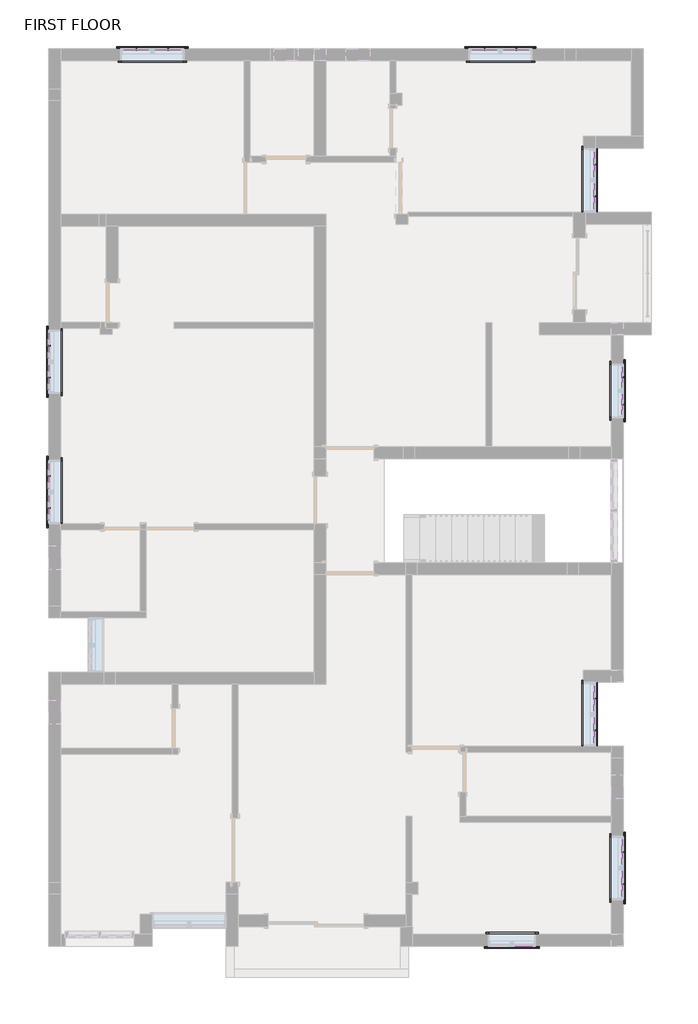
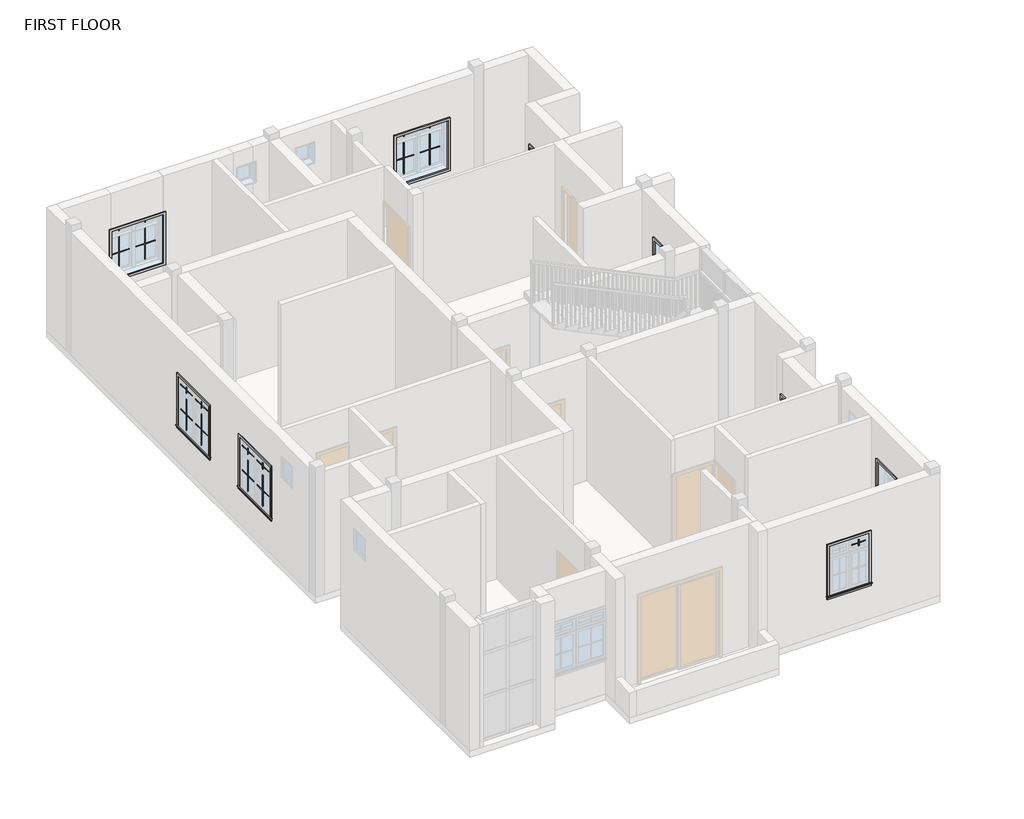
# One storey, part 6 of 6: 51 proxies.
"""IFC4 building model written with IfcOpenShell, lengths in millimetres."""

from ifc_helpers import new_model, si_unit, origin, place, context, project, spatial, transform, mapped, element, save
from components import muntin_pattern_2x2_muntin_pattern_2x2_2357e71d, muntin_pattern_2x2_muntin_pattern_2x2_302d8f29, muntin_pattern_2x2_muntin_pattern_2x2_3df65231, muntin_pattern_2x2_muntin_pattern_2x2_4af9dbf3, muntin_pattern_2x2_muntin_pattern_2x2_972acb6d, muntin_pattern_2x2_muntin_pattern_2x2_4879a4f3, muntin_pattern_2x2_muntin_pattern_2x2_604ffb00, trim_window_exterior_flat_with_sill_7cfdd449, trim_window_exterior_flat_with_sill_29d7a895, trim_window_exterior_flat_with_sill_e4b28ec3, trim_window_interior_flat_picture_frame_f1e0b15b, trim_window_interior_flat_picture_frame_56711e78, trim_window_interior_flat_picture_frame_39ff4276

model = new_model("IFC4")

# Units and contexts
model_context = context("Model", 3, world=origin())
ifc_project = project(units=[si_unit("LENGTHUNIT", "METRE", prefix="MILLI")], contexts=[model_context])

# Site, building, storey
site = spatial("IfcSite", under=ifc_project)
building = spatial("IfcBuilding", under=site)
storey = spatial("IfcBuildingStorey", under=building, Name="FIRST FLOOR", Elevation=3200.4)

# Proxies
placement = place(None, origin())
muntin_pattern_2x2_muntin_pattern_2x2_shape = muntin_pattern_2x2_muntin_pattern_2x2_2357e71d(model_context)
element("IfcBuildingElementProxy", 1, Name="Muntin Pattern_2x2 : Muntin Pattern_2x2", ObjectType="Muntin Pattern_2x2 : Muntin Pattern_2x2", at=placement, inside=storey, context=model_context, shape_type="MappedRepresentation", body=[
    mapped(muntin_pattern_2x2_muntin_pattern_2x2_shape, transform((-5090.4990981, 9290.6537587, 4184.65), x_axis=(1.0, 0.0, 0.0), y_axis=(0.0, 1.0, 0.0), z_axis=(0.0, 0.0, 1.0))),
])
element("IfcBuildingElementProxy", 2, Name="Muntin Pattern_2x2 : Muntin Pattern_2x2", ObjectType="Muntin Pattern_2x2 : Muntin Pattern_2x2", at=placement, inside=storey, context=model_context, shape_type="MappedRepresentation", body=[
    mapped(muntin_pattern_2x2_muntin_pattern_2x2_shape, transform((3661.3884019, 7088.7912587, 4184.65), x_axis=(0.0, -1.0, 0.0), y_axis=(1.0, 0.0, 0.0), z_axis=(0.0, 0.0, 1.0))),
])
element("IfcBuildingElementProxy", 3, Name="Muntin Pattern_2x2 : Muntin Pattern_2x2", ObjectType="Muntin Pattern_2x2 : Muntin Pattern_2x2", at=placement, inside=storey, context=model_context, shape_type="MappedRepresentation", body=[
    mapped(muntin_pattern_2x2_muntin_pattern_2x2_shape, transform((3661.3884019, -3096.6087413, 4184.65), x_axis=(0.0, -1.0, 0.0), y_axis=(1.0, 0.0, 0.0), z_axis=(0.0, 0.0, 1.0))),
])
element("IfcBuildingElementProxy", 4, Name="Muntin Pattern_2x2 : Muntin Pattern_2x2", ObjectType="Muntin Pattern_2x2 : Muntin Pattern_2x2", at=placement, inside=storey, context=model_context, shape_type="MappedRepresentation", body=[
    mapped(muntin_pattern_2x2_muntin_pattern_2x2_shape, transform((4194.7884019, -6025.7255734, 4184.65), x_axis=(0.0, -1.0, 0.0), y_axis=(1.0, 0.0, 0.0), z_axis=(0.0, 0.0, 1.0))),
])
element("IfcBuildingElementProxy", 5, Name="Muntin Pattern_2x2 : Muntin Pattern_2x2", ObjectType="Muntin Pattern_2x2 : Muntin Pattern_2x2", at=placement, inside=storey, context=model_context, shape_type="MappedRepresentation", body=[
    mapped(muntin_pattern_2x2_muntin_pattern_2x2_shape, transform((-6758.9615981, 538.7662587, 4184.65), x_axis=(0.0, 1.0, 0.0), y_axis=(-1.0, 0.0, 0.0), z_axis=(0.0, 0.0, 1.0))),
])
element("IfcBuildingElementProxy", 6, Name="Muntin Pattern_2x2 : Muntin Pattern_2x2", ObjectType="Muntin Pattern_2x2 : Muntin Pattern_2x2", at=placement, inside=storey, context=model_context, shape_type="MappedRepresentation", body=[
    mapped(muntin_pattern_2x2_muntin_pattern_2x2_shape, transform((-6758.9615981, 3024.5447861, 4184.65), x_axis=(0.0, 1.0, 0.0), y_axis=(-1.0, 0.0, 0.0), z_axis=(0.0, 0.0, 1.0))),
])
element("IfcBuildingElementProxy", 7, Name="Muntin Pattern_2x2 : Muntin Pattern_2x2", ObjectType="Muntin Pattern_2x2 : Muntin Pattern_2x2", at=placement, inside=storey, context=model_context, shape_type="MappedRepresentation", body=[
    mapped(muntin_pattern_2x2_muntin_pattern_2x2_shape, transform((1554.8452655, 9290.6537587, 4184.65), x_axis=(1.0, 0.0, 0.0), y_axis=(0.0, 1.0, 0.0), z_axis=(0.0, 0.0, 1.0))),
])
muntin_pattern_2x2_muntin_pattern_2x2_2_shape = muntin_pattern_2x2_muntin_pattern_2x2_302d8f29(model_context)
element("IfcBuildingElementProxy", 8, Name="Muntin Pattern_2x2 : Muntin Pattern_2x2", ObjectType="Muntin Pattern_2x2 : Muntin Pattern_2x2", at=placement, inside=storey, context=model_context, shape_type="MappedRepresentation", body=[
    mapped(muntin_pattern_2x2_muntin_pattern_2x2_2_shape, transform((-4484.0740981, 9290.6537587, 4184.65), x_axis=(-1.0, 0.0, 0.0), y_axis=(0.0, -1.0, 0.0), z_axis=(0.0, 0.0, 1.0))),
])
element("IfcBuildingElementProxy", 9, Name="Muntin Pattern_2x2 : Muntin Pattern_2x2", ObjectType="Muntin Pattern_2x2 : Muntin Pattern_2x2", at=placement, inside=storey, context=model_context, shape_type="MappedRepresentation", body=[
    mapped(muntin_pattern_2x2_muntin_pattern_2x2_2_shape, transform((3661.3884019, 6482.3662587, 4184.65), x_axis=(0.0, 1.0, 0.0), y_axis=(-1.0, 0.0, 0.0), z_axis=(0.0, 0.0, 1.0))),
])
element("IfcBuildingElementProxy", 10, Name="Muntin Pattern_2x2 : Muntin Pattern_2x2", ObjectType="Muntin Pattern_2x2 : Muntin Pattern_2x2", at=placement, inside=storey, context=model_context, shape_type="MappedRepresentation", body=[
    mapped(muntin_pattern_2x2_muntin_pattern_2x2_2_shape, transform((3661.3884019, -3703.0337413, 4184.65), x_axis=(0.0, 1.0, 0.0), y_axis=(-1.0, 0.0, 0.0), z_axis=(0.0, 0.0, 1.0))),
])
element("IfcBuildingElementProxy", 11, Name="Muntin Pattern_2x2 : Muntin Pattern_2x2", ObjectType="Muntin Pattern_2x2 : Muntin Pattern_2x2", at=placement, inside=storey, context=model_context, shape_type="MappedRepresentation", body=[
    mapped(muntin_pattern_2x2_muntin_pattern_2x2_2_shape, transform((4194.7884019, -6632.1505734, 4184.65), x_axis=(0.0, 1.0, 0.0), y_axis=(-1.0, 0.0, 0.0), z_axis=(0.0, 0.0, 1.0))),
])
element("IfcBuildingElementProxy", 12, Name="Muntin Pattern_2x2 : Muntin Pattern_2x2", ObjectType="Muntin Pattern_2x2 : Muntin Pattern_2x2", at=placement, inside=storey, context=model_context, shape_type="MappedRepresentation", body=[
    mapped(muntin_pattern_2x2_muntin_pattern_2x2_2_shape, transform((-6758.9615981, 1145.1912587, 4184.65), x_axis=(0.0, -1.0, 0.0), y_axis=(1.0, 0.0, 0.0), z_axis=(0.0, 0.0, 1.0))),
])
element("IfcBuildingElementProxy", 13, Name="Muntin Pattern_2x2 : Muntin Pattern_2x2", ObjectType="Muntin Pattern_2x2 : Muntin Pattern_2x2", at=placement, inside=storey, context=model_context, shape_type="MappedRepresentation", body=[
    mapped(muntin_pattern_2x2_muntin_pattern_2x2_2_shape, transform((-6758.9615981, 3630.9697861, 4184.65), x_axis=(0.0, -1.0, 0.0), y_axis=(1.0, 0.0, 0.0), z_axis=(0.0, 0.0, 1.0))),
])
element("IfcBuildingElementProxy", 14, Name="Muntin Pattern_2x2 : Muntin Pattern_2x2", ObjectType="Muntin Pattern_2x2 : Muntin Pattern_2x2", at=placement, inside=storey, context=model_context, shape_type="MappedRepresentation", body=[
    mapped(muntin_pattern_2x2_muntin_pattern_2x2_2_shape, transform((2161.2702655, 9290.6537587, 4184.65), x_axis=(-1.0, 0.0, 0.0), y_axis=(0.0, -1.0, 0.0), z_axis=(0.0, 0.0, 1.0))),
])
muntin_pattern_2x2_muntin_pattern_2x2_3_shape = muntin_pattern_2x2_muntin_pattern_2x2_3df65231(model_context)
element("IfcBuildingElementProxy", 15, Name="Muntin Pattern_2x2 : Muntin Pattern_2x2", ObjectType="Muntin Pattern_2x2 : Muntin Pattern_2x2", at=placement, inside=storey, context=model_context, shape_type="MappedRepresentation", body=[
    mapped(muntin_pattern_2x2_muntin_pattern_2x2_3_shape, transform((-4484.0740981, 9290.6537587, 5099.05), x_axis=(-1.0, 0.0, 0.0), y_axis=(0.0, -1.0, 0.0), z_axis=(0.0, 0.0, 1.0))),
])
element("IfcBuildingElementProxy", 16, Name="Muntin Pattern_2x2 : Muntin Pattern_2x2", ObjectType="Muntin Pattern_2x2 : Muntin Pattern_2x2", at=placement, inside=storey, context=model_context, shape_type="MappedRepresentation", body=[
    mapped(muntin_pattern_2x2_muntin_pattern_2x2_3_shape, transform((-5090.4990981, 9290.6537587, 5099.05), x_axis=(-1.0, 0.0, 0.0), y_axis=(0.0, -1.0, 0.0), z_axis=(0.0, 0.0, 1.0))),
])
element("IfcBuildingElementProxy", 17, Name="Muntin Pattern_2x2 : Muntin Pattern_2x2", ObjectType="Muntin Pattern_2x2 : Muntin Pattern_2x2", at=placement, inside=storey, context=model_context, shape_type="MappedRepresentation", body=[
    mapped(muntin_pattern_2x2_muntin_pattern_2x2_3_shape, transform((3661.3884019, 6482.3662587, 5099.05), x_axis=(0.0, 1.0, 0.0), y_axis=(-1.0, 0.0, 0.0), z_axis=(0.0, 0.0, 1.0))),
])
element("IfcBuildingElementProxy", 18, Name="Muntin Pattern_2x2 : Muntin Pattern_2x2", ObjectType="Muntin Pattern_2x2 : Muntin Pattern_2x2", at=placement, inside=storey, context=model_context, shape_type="MappedRepresentation", body=[
    mapped(muntin_pattern_2x2_muntin_pattern_2x2_3_shape, transform((3661.3884019, 7088.7912587, 5099.05), x_axis=(0.0, 1.0, 0.0), y_axis=(-1.0, 0.0, 0.0), z_axis=(0.0, 0.0, 1.0))),
])
element("IfcBuildingElementProxy", 19, Name="Muntin Pattern_2x2 : Muntin Pattern_2x2", ObjectType="Muntin Pattern_2x2 : Muntin Pattern_2x2", at=placement, inside=storey, context=model_context, shape_type="MappedRepresentation", body=[
    mapped(muntin_pattern_2x2_muntin_pattern_2x2_3_shape, transform((3661.3884019, -3703.0337413, 5099.05), x_axis=(0.0, 1.0, 0.0), y_axis=(-1.0, 0.0, 0.0), z_axis=(0.0, 0.0, 1.0))),
])
element("IfcBuildingElementProxy", 20, Name="Muntin Pattern_2x2 : Muntin Pattern_2x2", ObjectType="Muntin Pattern_2x2 : Muntin Pattern_2x2", at=placement, inside=storey, context=model_context, shape_type="MappedRepresentation", body=[
    mapped(muntin_pattern_2x2_muntin_pattern_2x2_3_shape, transform((3661.3884019, -3096.6087413, 5099.05), x_axis=(0.0, 1.0, 0.0), y_axis=(-1.0, 0.0, 0.0), z_axis=(0.0, 0.0, 1.0))),
])
element("IfcBuildingElementProxy", 21, Name="Muntin Pattern_2x2 : Muntin Pattern_2x2", ObjectType="Muntin Pattern_2x2 : Muntin Pattern_2x2", at=placement, inside=storey, context=model_context, shape_type="MappedRepresentation", body=[
    mapped(muntin_pattern_2x2_muntin_pattern_2x2_3_shape, transform((4194.7884019, -6632.1505734, 5099.05), x_axis=(0.0, 1.0, 0.0), y_axis=(-1.0, 0.0, 0.0), z_axis=(0.0, 0.0, 1.0))),
])
element("IfcBuildingElementProxy", 22, Name="Muntin Pattern_2x2 : Muntin Pattern_2x2", ObjectType="Muntin Pattern_2x2 : Muntin Pattern_2x2", at=placement, inside=storey, context=model_context, shape_type="MappedRepresentation", body=[
    mapped(muntin_pattern_2x2_muntin_pattern_2x2_3_shape, transform((4194.7884019, -6025.7255734, 5099.05), x_axis=(0.0, 1.0, 0.0), y_axis=(-1.0, 0.0, 0.0), z_axis=(0.0, 0.0, 1.0))),
])
element("IfcBuildingElementProxy", 23, Name="Muntin Pattern_2x2 : Muntin Pattern_2x2", ObjectType="Muntin Pattern_2x2 : Muntin Pattern_2x2", at=placement, inside=storey, context=model_context, shape_type="MappedRepresentation", body=[
    mapped(muntin_pattern_2x2_muntin_pattern_2x2_3_shape, transform((-6758.9615981, 1145.1912587, 5099.05), x_axis=(0.0, -1.0, 0.0), y_axis=(1.0, 0.0, 0.0), z_axis=(0.0, 0.0, 1.0))),
])
element("IfcBuildingElementProxy", 24, Name="Muntin Pattern_2x2 : Muntin Pattern_2x2", ObjectType="Muntin Pattern_2x2 : Muntin Pattern_2x2", at=placement, inside=storey, context=model_context, shape_type="MappedRepresentation", body=[
    mapped(muntin_pattern_2x2_muntin_pattern_2x2_3_shape, transform((-6758.9615981, 538.7662587, 5099.05), x_axis=(0.0, -1.0, 0.0), y_axis=(1.0, 0.0, 0.0), z_axis=(0.0, 0.0, 1.0))),
])
element("IfcBuildingElementProxy", 25, Name="Muntin Pattern_2x2 : Muntin Pattern_2x2", ObjectType="Muntin Pattern_2x2 : Muntin Pattern_2x2", at=placement, inside=storey, context=model_context, shape_type="MappedRepresentation", body=[
    mapped(muntin_pattern_2x2_muntin_pattern_2x2_3_shape, transform((-6758.9615981, 3630.9697861, 5099.05), x_axis=(0.0, -1.0, 0.0), y_axis=(1.0, 0.0, 0.0), z_axis=(0.0, 0.0, 1.0))),
])
element("IfcBuildingElementProxy", 26, Name="Muntin Pattern_2x2 : Muntin Pattern_2x2", ObjectType="Muntin Pattern_2x2 : Muntin Pattern_2x2", at=placement, inside=storey, context=model_context, shape_type="MappedRepresentation", body=[
    mapped(muntin_pattern_2x2_muntin_pattern_2x2_3_shape, transform((-6758.9615981, 3024.5447861, 5099.05), x_axis=(0.0, -1.0, 0.0), y_axis=(1.0, 0.0, 0.0), z_axis=(0.0, 0.0, 1.0))),
])
element("IfcBuildingElementProxy", 27, Name="Muntin Pattern_2x2 : Muntin Pattern_2x2", ObjectType="Muntin Pattern_2x2 : Muntin Pattern_2x2", at=placement, inside=storey, context=model_context, shape_type="MappedRepresentation", body=[
    mapped(muntin_pattern_2x2_muntin_pattern_2x2_3_shape, transform((2161.2702655, 9290.6537587, 5099.05), x_axis=(-1.0, 0.0, 0.0), y_axis=(0.0, -1.0, 0.0), z_axis=(0.0, 0.0, 1.0))),
])
element("IfcBuildingElementProxy", 28, Name="Muntin Pattern_2x2 : Muntin Pattern_2x2", ObjectType="Muntin Pattern_2x2 : Muntin Pattern_2x2", at=placement, inside=storey, context=model_context, shape_type="MappedRepresentation", body=[
    mapped(muntin_pattern_2x2_muntin_pattern_2x2_3_shape, transform((1554.8452655, 9290.6537587, 5099.05), x_axis=(-1.0, 0.0, 0.0), y_axis=(0.0, -1.0, 0.0), z_axis=(0.0, 0.0, 1.0))),
])
muntin_pattern_2x2_muntin_pattern_2x2_4_shape = muntin_pattern_2x2_muntin_pattern_2x2_4af9dbf3(model_context)
element("IfcBuildingElementProxy", 29, Name="Muntin Pattern_2x2 : Muntin Pattern_2x2", ObjectType="Muntin Pattern_2x2 : Muntin Pattern_2x2", at=placement, inside=storey, context=model_context, shape_type="MappedRepresentation", body=[
    mapped(muntin_pattern_2x2_muntin_pattern_2x2_4_shape, transform((4194.7884019, 3031.1412587, 4184.65), x_axis=(0.0, -1.0, 0.0), y_axis=(1.0, 0.0, 0.0), z_axis=(0.0, 0.0, 1.0))),
])
muntin_pattern_2x2_muntin_pattern_2x2_5_shape = muntin_pattern_2x2_muntin_pattern_2x2_972acb6d(model_context)
element("IfcBuildingElementProxy", 30, Name="Muntin Pattern_2x2 : Muntin Pattern_2x2", ObjectType="Muntin Pattern_2x2 : Muntin Pattern_2x2", at=placement, inside=storey, context=model_context, shape_type="MappedRepresentation", body=[
    mapped(muntin_pattern_2x2_muntin_pattern_2x2_5_shape, transform((4194.7884019, 2513.6162587, 4184.65), x_axis=(0.0, 1.0, 0.0), y_axis=(-1.0, 0.0, 0.0), z_axis=(0.0, 0.0, 1.0))),
])
muntin_pattern_2x2_muntin_pattern_2x2_6_shape = muntin_pattern_2x2_muntin_pattern_2x2_4879a4f3(model_context)
element("IfcBuildingElementProxy", 31, Name="Muntin Pattern_2x2 : Muntin Pattern_2x2", ObjectType="Muntin Pattern_2x2 : Muntin Pattern_2x2", at=placement, inside=storey, context=model_context, shape_type="MappedRepresentation", body=[
    mapped(muntin_pattern_2x2_muntin_pattern_2x2_6_shape, transform((4194.7884019, 2513.6162587, 5099.05), x_axis=(0.0, 1.0, 0.0), y_axis=(-1.0, 0.0, 0.0), z_axis=(0.0, 0.0, 1.0))),
])
element("IfcBuildingElementProxy", 32, Name="Muntin Pattern_2x2 : Muntin Pattern_2x2", ObjectType="Muntin Pattern_2x2 : Muntin Pattern_2x2", at=placement, inside=storey, context=model_context, shape_type="MappedRepresentation", body=[
    mapped(muntin_pattern_2x2_muntin_pattern_2x2_6_shape, transform((4194.7884019, 3031.1412587, 5099.05), x_axis=(0.0, 1.0, 0.0), y_axis=(-1.0, 0.0, 0.0), z_axis=(0.0, 0.0, 1.0))),
])
muntin_pattern_2x2_muntin_pattern_2x2_7_shape = muntin_pattern_2x2_muntin_pattern_2x2_604ffb00(model_context)
element("IfcBuildingElementProxy", 33, Name="Muntin Pattern_2x2 : Muntin Pattern_2x2", ObjectType="Muntin Pattern_2x2 : Muntin Pattern_2x2", at=placement, inside=storey, context=model_context, shape_type="MappedRepresentation", body=[
    mapped(muntin_pattern_2x2_muntin_pattern_2x2_7_shape, transform((2304.0759019, -7809.8962413, 5099.05), x_axis=(1.0, 0.0, 0.0), y_axis=(0.0, 1.0, 0.0), z_axis=(0.0, 0.0, 1.0))),
])
trim_window_exterior_flat_with_sill_shape = trim_window_exterior_flat_with_sill_7cfdd449(model_context)
element("IfcBuildingElementProxy", 34, Name="Trim-Window-Exterior-Flat : with Sill", ObjectType="Trim-Window-Exterior-Flat : with Sill", at=placement, inside=storey, context=model_context, shape_type="MappedRepresentation", body=[
    mapped(trim_window_exterior_flat_with_sill_shape, transform((-4787.2865981, 9300.1787587, 5334.0), x_axis=(-1.0, 0.0, 0.0), y_axis=(0.0, 0.0, 1.0), z_axis=(0.0, 1.0, 0.0))),
])
element("IfcBuildingElementProxy", 35, Name="Trim-Window-Exterior-Flat : with Sill", ObjectType="Trim-Window-Exterior-Flat : with Sill", at=placement, inside=storey, context=model_context, shape_type="MappedRepresentation", body=[
    mapped(trim_window_exterior_flat_with_sill_shape, transform((3670.9134019, 6785.5787587, 5334.0), x_axis=(0.0, 1.0, 0.0), y_axis=(0.0, 0.0, 1.0), z_axis=(1.0, 0.0, 0.0))),
])
element("IfcBuildingElementProxy", 36, Name="Trim-Window-Exterior-Flat : with Sill", ObjectType="Trim-Window-Exterior-Flat : with Sill", at=placement, inside=storey, context=model_context, shape_type="MappedRepresentation", body=[
    mapped(trim_window_exterior_flat_with_sill_shape, transform((3670.9134019, -3399.8212413, 5334.0), x_axis=(0.0, 1.0, 0.0), y_axis=(0.0, 0.0, 1.0), z_axis=(1.0, 0.0, 0.0))),
])
element("IfcBuildingElementProxy", 37, Name="Trim-Window-Exterior-Flat : with Sill", ObjectType="Trim-Window-Exterior-Flat : with Sill", at=placement, inside=storey, context=model_context, shape_type="MappedRepresentation", body=[
    mapped(trim_window_exterior_flat_with_sill_shape, transform((4204.3134019, -6328.9380734, 5334.0), x_axis=(0.0, 1.0, 0.0), y_axis=(0.0, 0.0, 1.0), z_axis=(1.0, 0.0, 0.0))),
])
element("IfcBuildingElementProxy", 38, Name="Trim-Window-Exterior-Flat : with Sill", ObjectType="Trim-Window-Exterior-Flat : with Sill", at=placement, inside=storey, context=model_context, shape_type="MappedRepresentation", body=[
    mapped(trim_window_exterior_flat_with_sill_shape, transform((-6768.4865981, 841.9787587, 5334.0), x_axis=(0.0, -1.0, 0.0), y_axis=(0.0, 0.0, 1.0), z_axis=(-1.0, 0.0, 0.0))),
])
element("IfcBuildingElementProxy", 39, Name="Trim-Window-Exterior-Flat : with Sill", ObjectType="Trim-Window-Exterior-Flat : with Sill", at=placement, inside=storey, context=model_context, shape_type="MappedRepresentation", body=[
    mapped(trim_window_exterior_flat_with_sill_shape, transform((-6768.4865981, 3327.7572861, 5334.0), x_axis=(0.0, -1.0, 0.0), y_axis=(0.0, 0.0, 1.0), z_axis=(-1.0, 0.0, 0.0))),
])
element("IfcBuildingElementProxy", 40, Name="Trim-Window-Exterior-Flat : with Sill", ObjectType="Trim-Window-Exterior-Flat : with Sill", at=placement, inside=storey, context=model_context, shape_type="MappedRepresentation", body=[
    mapped(trim_window_exterior_flat_with_sill_shape, transform((1858.0577655, 9300.1787587, 5334.0), x_axis=(-1.0, 0.0, 0.0), y_axis=(0.0, 0.0, 1.0), z_axis=(0.0, 1.0, 0.0))),
])
trim_window_exterior_flat_with_sill_2_shape = trim_window_exterior_flat_with_sill_29d7a895(model_context)
element("IfcBuildingElementProxy", 41, Name="Trim-Window-Exterior-Flat : with Sill", ObjectType="Trim-Window-Exterior-Flat : with Sill", at=placement, inside=storey, context=model_context, shape_type="MappedRepresentation", body=[
    mapped(trim_window_exterior_flat_with_sill_2_shape, transform((4204.3134019, 2772.3787587, 5334.0), x_axis=(0.0, 1.0, 0.0), y_axis=(0.0, 0.0, 1.0), z_axis=(1.0, 0.0, 0.0))),
])
trim_window_exterior_flat_with_sill_3_shape = trim_window_exterior_flat_with_sill_e4b28ec3(model_context)
element("IfcBuildingElementProxy", 42, Name="Trim-Window-Exterior-Flat : with Sill", ObjectType="Trim-Window-Exterior-Flat : with Sill", at=placement, inside=storey, context=model_context, shape_type="MappedRepresentation", body=[
    mapped(trim_window_exterior_flat_with_sill_3_shape, transform((2077.0634019, -7819.4212413, 5334.0), x_axis=(1.0, 0.0, 0.0), y_axis=(0.0, 0.0, 1.0), z_axis=(0.0, -1.0, 0.0))),
])
trim_window_interior_flat_picture_frame_shape = trim_window_interior_flat_picture_frame_f1e0b15b(model_context)
element("IfcBuildingElementProxy", 43, Name="Trim-Window-Interior-Flat : Picture Frame", ObjectType="Trim-Window-Interior-Flat : Picture Frame", at=placement, inside=storey, context=model_context, shape_type="MappedRepresentation", body=[
    mapped(trim_window_interior_flat_picture_frame_shape, transform((-4787.2865981, 9071.5787587, 5334.0), x_axis=(1.0, 0.0, 0.0), y_axis=(0.0, 0.0, 1.0), z_axis=(0.0, -1.0, 0.0))),
])
element("IfcBuildingElementProxy", 44, Name="Trim-Window-Interior-Flat : Picture Frame", ObjectType="Trim-Window-Interior-Flat : Picture Frame", at=placement, inside=storey, context=model_context, shape_type="MappedRepresentation", body=[
    mapped(trim_window_interior_flat_picture_frame_shape, transform((3442.3134019, 6785.5787587, 5334.0), x_axis=(0.0, -1.0, 0.0), y_axis=(0.0, 0.0, 1.0), z_axis=(-1.0, 0.0, 0.0))),
])
element("IfcBuildingElementProxy", 45, Name="Trim-Window-Interior-Flat : Picture Frame", ObjectType="Trim-Window-Interior-Flat : Picture Frame", at=placement, inside=storey, context=model_context, shape_type="MappedRepresentation", body=[
    mapped(trim_window_interior_flat_picture_frame_shape, transform((3442.3134019, -3399.8212413, 5334.0), x_axis=(0.0, -1.0, 0.0), y_axis=(0.0, 0.0, 1.0), z_axis=(-1.0, 0.0, 0.0))),
])
element("IfcBuildingElementProxy", 46, Name="Trim-Window-Interior-Flat : Picture Frame", ObjectType="Trim-Window-Interior-Flat : Picture Frame", at=placement, inside=storey, context=model_context, shape_type="MappedRepresentation", body=[
    mapped(trim_window_interior_flat_picture_frame_shape, transform((3975.7134019, -6328.9380734, 5334.0), x_axis=(0.0, -1.0, 0.0), y_axis=(0.0, 0.0, 1.0), z_axis=(-1.0, 0.0, 0.0))),
])
element("IfcBuildingElementProxy", 47, Name="Trim-Window-Interior-Flat : Picture Frame", ObjectType="Trim-Window-Interior-Flat : Picture Frame", at=placement, inside=storey, context=model_context, shape_type="MappedRepresentation", body=[
    mapped(trim_window_interior_flat_picture_frame_shape, transform((-6539.8865981, 841.9787587, 5334.0), x_axis=(0.0, 1.0, 0.0), y_axis=(0.0, 0.0, 1.0), z_axis=(1.0, 0.0, 0.0))),
])
element("IfcBuildingElementProxy", 48, Name="Trim-Window-Interior-Flat : Picture Frame", ObjectType="Trim-Window-Interior-Flat : Picture Frame", at=placement, inside=storey, context=model_context, shape_type="MappedRepresentation", body=[
    mapped(trim_window_interior_flat_picture_frame_shape, transform((-6539.8865981, 3327.7572861, 5334.0), x_axis=(0.0, 1.0, 0.0), y_axis=(0.0, 0.0, 1.0), z_axis=(1.0, 0.0, 0.0))),
])
element("IfcBuildingElementProxy", 49, Name="Trim-Window-Interior-Flat : Picture Frame", ObjectType="Trim-Window-Interior-Flat : Picture Frame", at=placement, inside=storey, context=model_context, shape_type="MappedRepresentation", body=[
    mapped(trim_window_interior_flat_picture_frame_shape, transform((1858.0577655, 9071.5787587, 5334.0), x_axis=(1.0, 0.0, 0.0), y_axis=(0.0, 0.0, 1.0), z_axis=(0.0, -1.0, 0.0))),
])
trim_window_interior_flat_picture_frame_2_shape = trim_window_interior_flat_picture_frame_56711e78(model_context)
element("IfcBuildingElementProxy", 50, Name="Trim-Window-Interior-Flat : Picture Frame", ObjectType="Trim-Window-Interior-Flat : Picture Frame", at=placement, inside=storey, context=model_context, shape_type="MappedRepresentation", body=[
    mapped(trim_window_interior_flat_picture_frame_2_shape, transform((3975.7134019, 2772.3787587, 5334.0), x_axis=(0.0, -1.0, 0.0), y_axis=(0.0, 0.0, 1.0), z_axis=(-1.0, 0.0, 0.0))),
])
trim_window_interior_flat_picture_frame_3_shape = trim_window_interior_flat_picture_frame_39ff4276(model_context)
element("IfcBuildingElementProxy", 51, Name="Trim-Window-Interior-Flat : Picture Frame", ObjectType="Trim-Window-Interior-Flat : Picture Frame", at=placement, inside=storey, context=model_context, shape_type="MappedRepresentation", body=[
    mapped(trim_window_interior_flat_picture_frame_3_shape, transform((2077.0634019, -7590.8212413, 5334.0), x_axis=(-1.0, 0.0, 0.0), y_axis=(0.0, 0.0, 1.0), z_axis=(0.0, 1.0, 0.0))),
])

save(model, "model.ifc")

# Revit data of these elements
# Type "Muntin Pattern_2x2 : Muntin Pattern_2x2"
#   Width [instance default] = 4' - 0"
#   Thickness = 0' - 0 1/2"
#   Height [instance default] = 4' - 0"
#   Distance = 0' - 0 3/4"
#   Interior Material [instance default] = none
#   Exterior Material [instance default] = none
#   Default Elevation = 0
# Type "Trim-Window-Exterior-Flat : with Sill"
#   Trim Width = 0' - 2 1/4"
#   Trim Thickness_Picture Frame = 0' - 1 1/4"
#   Trim Thickness_with Sill = 0' - 0 3/4"
#   Sill Thickness = 0' - 1 1/4"
#   Opening Width [instance default] = 2' - 0"
#   Opening Height [instance default] = 3' - 0"
#   Default Elevation = 4' - 0"
#   Sill = yes
#   Picture Frame = no
#   Trim Material [instance default] = none
# Type "Trim-Window-Interior-Flat : Picture Frame"
#   Trim Thickness_Picture Frame = 0' - 1 1/4"
#   Trim Width = 0' - 2 1/4"
#   Trim Thickness_with Sill = 0' - 0 3/4"
#   Sill Thickness = 0' - 1 1/4"
#   Opening Width [instance default] = 2' - 0"
#   Opening Height [instance default] = 3' - 0"
#   Default Elevation = 4' - 0"
#   Sill = no
#   Picture Frame = yes
#   Trim Material [instance default] = none
# Elements 1, 2, 3, 4, 5, 6, 7, 8, 9, 10, 11, 12, 13, 14 (IfcBuildingElementProxy, "Muntin Pattern_2x2 : Muntin Pattern_2x2")
#   Width = 1' - 6 5/8"
#   Height = 2' - 6 1/2"
#   Interior Material = Wood - Stained
#   Exterior Material = Clad - White
#   Phase Created = New Construction
#   Materials on its faces: "Clad - White", "Wood - Stained"
# Elements 15, 16, 17, 18, 19, 20, 21, 22, 23, 24, 25, 26, 27, 28 (IfcBuildingElementProxy, "Muntin Pattern_2x2 : Muntin Pattern_2x2")
#   Width = 1' - 6 5/8"
#   Height = 0' - 6 1/2"
#   Interior Material = Wood - Stained
#   Exterior Material = Clad - White
#   Phase Created = New Construction
#   Materials on its faces: "Clad - White", "Wood - Stained"
# Elements 29, 30 (IfcBuildingElementProxy, "Muntin Pattern_2x2 : Muntin Pattern_2x2")
#   Width = 1' - 3 1/8"
#   Height = 2' - 6 1/2"
#   Interior Material = Wood - Stained
#   Exterior Material = Clad - White
#   Phase Created = New Construction
#   Materials on its faces: "Clad - White", "Wood - Stained"
# Elements 31, 32 (IfcBuildingElementProxy, "Muntin Pattern_2x2 : Muntin Pattern_2x2")
#   Width = 1' - 3 1/8"
#   Height = 0' - 6 1/2"
#   Interior Material = Wood - Stained
#   Exterior Material = Clad - White
#   Phase Created = New Construction
#   Materials on its faces: "Clad - White", "Wood - Stained"
# Element 33 (IfcBuildingElementProxy, "Muntin Pattern_2x2 : Muntin Pattern_2x2")
#   Width = 1' - 0 5/8"
#   Height = 0' - 6 1/2"
#   Interior Material = Wood - Stained
#   Exterior Material = Clad - White
#   Phase Created = New Construction
#   Materials on its faces: "Clad - White", "Wood - Stained"
# Elements 34, 35, 36, 37, 38, 39, 40 (IfcBuildingElementProxy, "Trim-Window-Exterior-Flat : with Sill")
#   Opening Width = 4' - 0"
#   Opening Height = 4' - 0"
#   Trim Material = Clad - White
#   Phase Created = New Construction
#   Materials on its faces: "Clad - White"
# Element 41 (IfcBuildingElementProxy, "Trim-Window-Exterior-Flat : with Sill")
#   Opening Width = 3' - 5"
#   Opening Height = 4' - 0"
#   Trim Material = Clad - White
#   Phase Created = New Construction
#   Materials on its faces: "Clad - White"
# Element 42 (IfcBuildingElementProxy, "Trim-Window-Exterior-Flat : with Sill")
#   Opening Width = 3' - 0"
#   Opening Height = 4' - 0"
#   Trim Material = Clad - White
#   Phase Created = New Construction
#   Materials on its faces: "Clad - White"
# Elements 43, 44, 45, 46, 47, 48, 49 (IfcBuildingElementProxy, "Trim-Window-Interior-Flat : Picture Frame")
#   Opening Width = 4' - 0"
#   Opening Height = 4' - 0"
#   Trim Material = Wood - Stained
#   Phase Created = New Construction
#   Materials on its faces: "Wood - Stained"
# Element 50 (IfcBuildingElementProxy, "Trim-Window-Interior-Flat : Picture Frame")
#   Opening Width = 3' - 5"
#   Opening Height = 4' - 0"
#   Trim Material = Wood - Stained
#   Phase Created = New Construction
#   Materials on its faces: "Wood - Stained"
# Element 51 (IfcBuildingElementProxy, "Trim-Window-Interior-Flat : Picture Frame")
#   Opening Width = 3' - 0"
#   Opening Height = 4' - 0"
#   Trim Material = Wood - Stained
#   Phase Created = New Construction
#   Materials on its faces: "Wood - Stained"
# Materials
#   "Clad - White": class "Wood", colour RGB 242 242 238, transparency 0, Cost = 0
#   "Wood - Stained": class "Wood", colour RGB 224 178 126, transparency 0, Cost = 0
